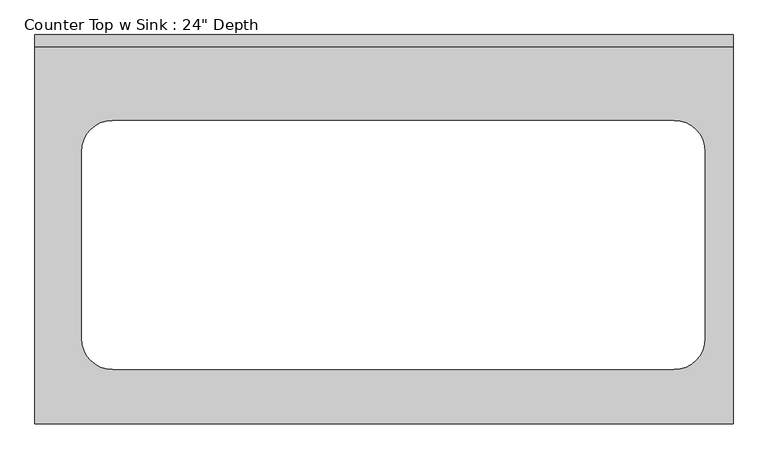
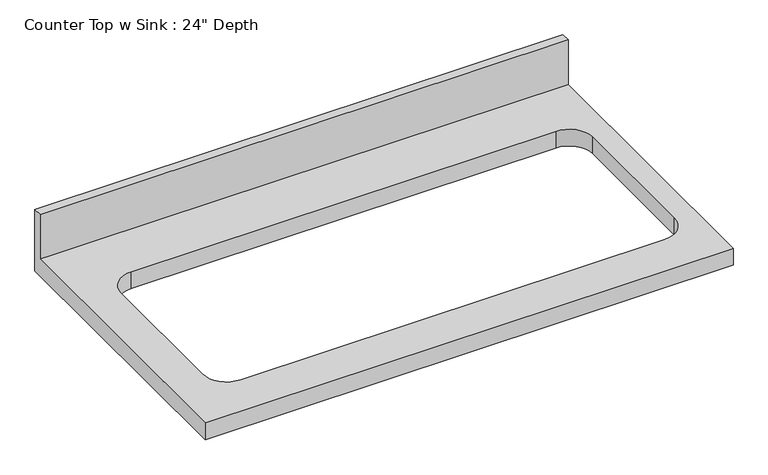
"""IFC4 building model written with IfcOpenShell, lengths in millimetres: furniture geometry."""

from ifc_helpers import new_model, si_unit, frame, origin, place, context, project, spatial, polyline, circle_curve, source, transform, mapped, element, save
from ifc_brep_helpers import plane_surface, revolved_surface, advanced_brep


def furniture_5f80dcf3(model_context):
    return source(origin(), model_context, "Body", "AdvancedBrep", [
        advanced_brep(
        [(-1200.4622951, -635.0, 914.4), (-62.4534477, -635.0, 914.4), (-62.4534477, -19.05, 914.4), (-1200.4622951, -19.05, 914.4), (-1073.4622951, -139.7, 914.4), (-159.0622951, -139.7, 914.4), (-108.2622951, -190.5, 914.4), (-108.2622951, -495.3, 914.4), (-159.0622951, -546.1, 914.4), (-1073.4622951, -546.1, 914.4), (-1124.2622951, -495.3, 914.4), (-1124.2622951, -190.5, 914.4), (-62.4534477, 0.0, 876.3), (-62.4534477, -635.0, 876.3), (-1200.4622951, -635.0, 876.3), (-1200.4622951, 0.0, 876.3), (-159.0622951, -139.7, 876.3), (-1073.4622951, -139.7, 876.3), (-1124.2622951, -190.5, 876.3), (-1124.2622951, -495.3, 876.3), (-1073.4622951, -546.1, 876.3), (-159.0622951, -546.1, 876.3), (-108.2622951, -495.3, 876.3), (-108.2622951, -190.5, 876.3), (-1200.4622951, 0.0, 1016.0), (-62.4534477, 0.0, 1016.0), (-1200.4622951, -19.05, 1016.0), (-62.4534477, -19.05, 1016.0)],
        [
            (0, 1),
            (1, 2),
            (2, 3),
            (3, 0),
            (4, 5),
            (5, 6, circle_curve(frame((-159.0622951, -190.5, 914.4), z_axis=(0.0, 0.0, -1.0), x_axis=(1.0, 0.0, 0.0)), 50.8)),
            (6, 7),
            (7, 8, circle_curve(frame((-159.0622951, -495.3, 914.4), z_axis=(0.0, 0.0, -1.0), x_axis=(1.0, 0.0, 0.0)), 50.8)),
            (8, 9),
            (9, 10, circle_curve(frame((-1073.4622951, -495.3, 914.4), z_axis=(0.0, 0.0, -1.0), x_axis=(1.0, 0.0, 0.0)), 50.8)),
            (10, 11),
            (11, 4, circle_curve(frame((-1073.4622951, -190.5, 914.4), z_axis=(0.0, 0.0, -1.0), x_axis=(1.0, 0.0, 0.0)), 50.8)),
            (12, 13),
            (13, 14),
            (14, 15),
            (15, 12),
            (16, 17),
            (17, 18, circle_curve(frame((-1073.4622951, -190.5, 876.3), z_axis=(0.0, 0.0, 1.0), x_axis=(1.0, 0.0, 0.0)), 50.8)),
            (18, 19),
            (19, 20, circle_curve(frame((-1073.4622951, -495.3, 876.3), z_axis=(0.0, 0.0, 1.0), x_axis=(1.0, 0.0, 0.0)), 50.8)),
            (20, 21),
            (21, 22, circle_curve(frame((-159.0622951, -495.3, 876.3), z_axis=(0.0, 0.0, 1.0), x_axis=(1.0, 0.0, 0.0)), 50.8)),
            (22, 23),
            (23, 16, circle_curve(frame((-159.0622951, -190.5, 876.3), z_axis=(0.0, 0.0, 1.0), x_axis=(1.0, 0.0, 0.0)), 50.8)),
            (15, 24),
            (24, 25),
            (25, 12),
            (14, 0),
            (3, 26),
            (26, 24),
            (13, 1),
            (25, 27),
            (27, 2),
            (26, 27),
            (4, 17),
            (16, 5),
            (11, 18),
            (10, 19),
            (9, 20),
            (8, 21),
            (7, 22),
            (6, 23),
        ],
        [
            plane_surface(frame((-1200.4622951, 0.0, 914.4), z_axis=(0.0, 0.0, 1.0), x_axis=(-1.0, 0.0, 0.0))),
            plane_surface(frame((-1200.4622951, 0.0, 876.3), z_axis=(0.0, 0.0, -1.0), x_axis=(1.0, 0.0, 0.0))),
            plane_surface(frame((-62.4534477, 0.0, 914.4), z_axis=(0.0, 1.0, 0.0), x_axis=(0.0, 0.0, -1.0))),
            plane_surface(frame((-1200.4622951, 0.0, 914.4), z_axis=(-1.0, 0.0, 0.0), x_axis=(0.0, 0.0, -1.0))),
            plane_surface(frame((-1200.4622951, -635.0, 914.4), z_axis=(0.0, -1.0, 0.0), x_axis=(0.0, 0.0, -1.0))),
            plane_surface(frame((-62.4534477, -635.0, 914.4), z_axis=(1.0, 0.0, 0.0), x_axis=(0.0, 0.0, -1.0))),
            plane_surface(frame((-1200.4622951, 0.0, 1016.0), z_axis=(0.0, 0.0, 1.0), x_axis=(0.0, -1.0, 0.0))),
            plane_surface(frame((-1200.4622951, -19.05, 1016.0), z_axis=(0.0, -1.0, 0.0), x_axis=(0.0, 0.0, -1.0))),
            plane_surface(frame((-159.0622951, -139.7, 914.4), z_axis=(0.0, -1.0, 0.0), x_axis=(0.0, 0.0, -1.0))),
            revolved_surface(polyline([(-1022.6622950999999, -190.5, 914.4), (-1022.6622950999999, -190.5, 876.3)]), (-1073.4622951, -190.5, 876.3), (0.0, 0.0, 1.0)),
            plane_surface(frame((-1124.2622951, -190.5, 914.4), z_axis=(1.0, 0.0, 0.0), x_axis=(0.0, 0.0, -1.0))),
            revolved_surface(polyline([(-1022.6622950999999, -495.3, 914.4), (-1022.6622950999999, -495.3, 876.3)]), (-1073.4622951, -495.3, 876.3), (0.0, 0.0, 1.0)),
            plane_surface(frame((-1073.4622951, -546.1, 914.4), z_axis=(0.0, 1.0, 0.0), x_axis=(0.0, 0.0, -1.0))),
            revolved_surface(polyline([(-108.2622951, -495.3, 914.4), (-108.2622951, -495.3, 876.3)]), (-159.0622951, -495.3, 876.3), (0.0, 0.0, 1.0)),
            plane_surface(frame((-108.2622951, -495.3, 914.4), z_axis=(-1.0, 0.0, 0.0), x_axis=(0.0, 0.0, -1.0))),
            revolved_surface(polyline([(-108.2622951, -190.5, 914.4), (-108.2622951, -190.5, 876.3)]), (-159.0622951, -190.5, 876.3), (0.0, 0.0, 1.0)),
        ],
        [
            (0, [[1, 2, 3, 4], [5, 6, 7, 8, 9, 10, 11, 12]]),
            (1, [[13, 14, 15, 16], [17, 18, 19, 20, 21, 22, 23, 24]]),
            (2, [[-16, 25, 26, 27]]),
            (3, [[-15, 28, -4, 29, 30, -25]]),
            (4, [[-1, -28, -14, 31]]),
            (5, [[-13, -27, 32, 33, -2, -31]]),
            (6, [[-30, 34, -32, -26]]),
            (7, [[-34, -29, -3, -33]]),
            (8, [[35, -17, 36, -5]]),
            (9, [[-35, -12, 37, -18]]),
            (10, [[-37, -11, 38, -19]]),
            (11, [[-38, -10, 39, -20]]),
            (12, [[-39, -9, 40, -21]]),
            (13, [[-40, -8, 41, -22]]),
            (14, [[-41, -7, 42, -23]]),
            (15, [[-36, -24, -42, -6]]),
        ],
    ),
    ])


if __name__ == "__main__":
    model = new_model("IFC4")
    model_context = context("Model", 3, world=origin())
    ifc_project = project(units=[si_unit("LENGTHUNIT", "METRE", prefix="MILLI")], contexts=[model_context])
    site = spatial("IfcSite", under=ifc_project)
    building = spatial("IfcBuilding", under=site)
    placement = place(None, origin())
    furniture_shape = furniture_5f80dcf3(model_context)
    element("IfcFurniture", 1, ObjectType="Counter Top w Sink : 24\" Depth", at=placement, inside=building, context=model_context, shape_type="MappedRepresentation", body=[
        mapped(furniture_shape, transform((0.0, 0.0, 0.0), x_axis=(1.0, 0.0, 0.0), y_axis=(0.0, 1.0, 0.0), z_axis=(0.0, 0.0, 1.0))),
    ])
    save(model, "model.ifc")

# Revit data of these elements
# Type "Counter Top w Sink : 24\" Depth"
#   Assembly Code = "C1030400"
#   Counter Thickness = 0' - 1 1/2"
#   Depth = 2' - 1"
#   Height = 3' - 0"
#   Length [instance default] = 8' - 0"
#   Sink Location [instance default] = 2' - 0"
#   Sink Location To Wall [instance default] = 0' - 6"
#   Sink Opening Depth [instance default] = 1' - 3"
#   Sink Opening Width [instance default] = 3' - 3"
#   Counter Top Material = none
#   Default Elevation = 0
# Element 1 (IfcFurniture, "Counter Top w Sink : 24\" Depth")
#   Length = 3' - 8.8035"
#   Sink Location = 1' - 11"
#   Materials on its faces: "Counter Top"
# Materials
#   "Counter Top": class "Wood", colour RGB 226 177 128, transparency 0
